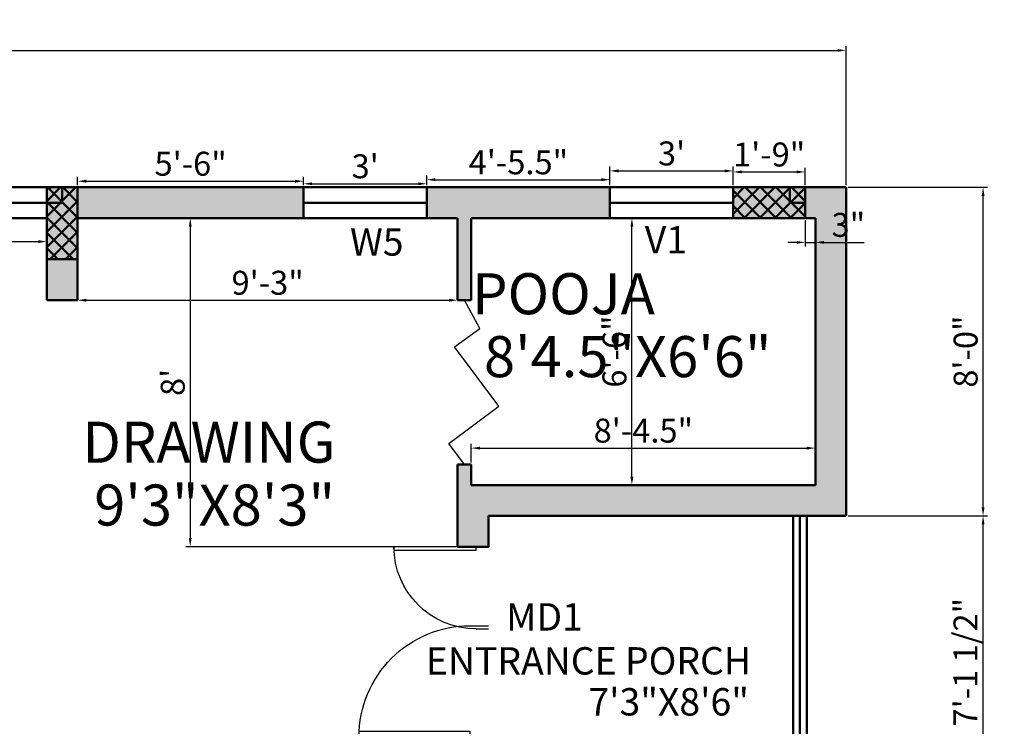
# Model space of a CAD drawing. Units: inches. Extents: x 1749 to 3550, y 1117 to 2383.
# Tile 5 of 15: x 2277 to 2565, y 1481 to 1687. Entities that reach past the tile are written whole.
import ezdxf

# ---------------------------------------------------------------- set-up
doc = ezdxf.new("R2010")
doc.units = ezdxf.units.IN
for name, color, linetype, lineweight in [('A-ANNO-DIMS', 2, 'Continuous', 18), ('A-ANNO-TEXT', 3, 'Continuous', 18), ('A-AREA-IDEN', 7, 'Continuous', 18), ('A-COLS', 10, 'Continuous', 50), ('A-DOOR', 30, 'Continuous', 25), ('A-WALL', 7, 'Continuous', 50), ('A-WALL-PATT', 8, 'Continuous', 13)]:
    doc.layers.add(name, color=color, linetype=linetype, lineweight=lineweight)
doc.styles.get("Standard").update_dxf_attribs({"font": 'arial.ttf'})
doc.dimstyles.new('ISO-25', dxfattribs={"dimtxt": 7, "dimasz": 2.5, "dimexe": 1.25, "dimexo": 0.625, "dimtad": 1, "dimdec": 1, "dimlunit": 3, "dimtxsty": 'Standard', "dimcen": 2.5, "dimadec": 0, "dimazin": 0, "dimtfac": 1, "dimtdec": 1, "dimtmove": 0, "dimatfit": 3, "dimfxl": 1, "dimarcsym": 0})

# ---------------------------------------------------------------- blocks, each defined once
blk = doc.blocks.new('*U14')
for p, q in [((0, 0), (0, 6)), ((36, 0), (36, 6))]:
    blk.add_line(p, q)
blk.add_lwpolyline([(0, 0), (0, -36), (1.75, -36), (1.75, 0)], close=True)
blk.add_arc((0, 0), 36, 270, 0)
blk = doc.blocks.new('*U13')
for p, q in [((0, 0), (0, -6)), ((40, 0), (40, -6))]:
    blk.add_line(p, q)
blk.add_lwpolyline([(0, 0), (0, 40), (1.75, 40), (1.75, 0)], close=True)
blk.add_arc((0, 0), 40, 0, 90)
blk = doc.blocks.new('*D17')
at = {"layer": 'A-ANNO-DIMS', "color": 0, "lineweight": -2, "ltscale": 0.5, "transparency": 16777216}
for p, q in [((2456.64, 1629.24), (2457.26, 1629.24)), ((2456.01, 1553.74), (2456.01, 1626.74)), ((2456.64, 1551.24), (2457.26, 1551.24))]:
    blk.add_line(p, q, dxfattribs=at)
at = {"layer": 'A-ANNO-DIMS', "color": 0, "ltscale": 0.5, "transparency": 16777216}
for points in [[(2455.6, 1626.74), (2456.43, 1626.74), (2456.01, 1629.24)], [(2455.6, 1553.74), (2456.43, 1553.74), (2456.01, 1551.24)]]:
    blk.add_solid(points, dxfattribs=at)
at = {"layer": 'Defpoints', "color": 0, "ltscale": 0.5, "transparency": 16777216}
for p in [(2456.01, 1629.24), (2456.01, 1629.24), (2456.01, 1551.24)]:
    blk.add_point(p, dxfattribs=at)
at = {"layer": 'A-ANNO-DIMS', "color": 0, "ltscale": 0.5, "transparency": 16777216, "insert": (2451.81, 1590.24), "char_height": 7, "attachment_point": 5, "rotation": 90}
blk.add_mtext('6\'-6"', dxfattribs=at)
blk = doc.blocks.new('*D18')
at = {"layer": 'A-ANNO-DIMS', "color": 0, "lineweight": -2, "ltscale": 0.5, "transparency": 16777216}
for p, q in [((2409.1, 1557.87), (2409.1, 1563.29)), ((2411.6, 1562.04), (2507.1, 1562.04)), ((2509.6, 1557.87), (2509.6, 1563.29))]:
    blk.add_line(p, q, dxfattribs=at)
at = {"layer": 'A-ANNO-DIMS', "color": 0, "ltscale": 0.5, "transparency": 16777216}
for points in [[(2411.6, 1562.46), (2411.6, 1561.62), (2409.1, 1562.04)], [(2507.1, 1562.46), (2507.1, 1561.62), (2509.6, 1562.04)]]:
    blk.add_solid(points, dxfattribs=at)
at = {"layer": 'Defpoints', "color": 0, "ltscale": 0.5, "transparency": 16777216}
for p in [(2509.6, 1562.04), (2409.1, 1557.24), (2509.6, 1557.24)]:
    blk.add_point(p, dxfattribs=at)
at = {"layer": 'A-ANNO-DIMS', "color": 0, "ltscale": 0.5, "transparency": 16777216, "insert": (2459.35, 1566.24), "char_height": 7, "attachment_point": 5}
blk.add_mtext('8\'-4.5"', dxfattribs=at)
blk = doc.blocks.new('*D30')
at = {"layer": 'A-ANNO-DIMS', "color": 0, "lineweight": -2, "ltscale": 0.5, "transparency": 16777216}
for p, q in [((2404.48, 1629.24), (2325.74, 1629.24)), ((2326.99, 1626.74), (2326.99, 1535.74)), ((2404.48, 1533.24), (2325.74, 1533.24))]:
    blk.add_line(p, q, dxfattribs=at)
at = {"layer": 'A-ANNO-DIMS', "color": 0, "ltscale": 0.5, "transparency": 16777216}
for points in [[(2326.58, 1626.74), (2327.41, 1626.74), (2326.99, 1629.24)], [(2326.58, 1535.74), (2327.41, 1535.74), (2326.99, 1533.24)]]:
    blk.add_solid(points, dxfattribs=at)
at = {"layer": 'Defpoints', "color": 0, "ltscale": 0.5, "transparency": 16777216}
for p in [(2405.1, 1629.24), (2326.99, 1533.24), (2405.1, 1533.24)]:
    blk.add_point(p, dxfattribs=at)
at = {"layer": 'A-ANNO-DIMS', "color": 0, "ltscale": 0.5, "transparency": 16777216, "insert": (2322.79, 1581.24), "char_height": 7, "attachment_point": 5, "rotation": 90}
blk.add_mtext("8'", dxfattribs=at)
blk = doc.blocks.new('*D31')
at = {"layer": 'A-ANNO-DIMS', "color": 0, "lineweight": -2, "ltscale": 0.5, "transparency": 16777216}
for p, q in [((2294.1, 1605.87), (2294.1, 1606.49)), ((2296.6, 1605.24), (2402.6, 1605.24)), ((2405.1, 1605.87), (2405.1, 1606.49))]:
    blk.add_line(p, q, dxfattribs=at)
at = {"layer": 'A-ANNO-DIMS', "color": 0, "ltscale": 0.5, "transparency": 16777216}
for points in [[(2296.6, 1605.66), (2296.6, 1604.83), (2294.1, 1605.24)], [(2402.6, 1605.66), (2402.6, 1604.83), (2405.1, 1605.24)]]:
    blk.add_solid(points, dxfattribs=at)
at = {"layer": 'Defpoints', "color": 0, "ltscale": 0.5, "transparency": 16777216}
for p in [(2294.1, 1605.24), (2405.1, 1605.24), (2405.1, 1605.24)]:
    blk.add_point(p, dxfattribs=at)
at = {"layer": 'A-ANNO-DIMS', "color": 0, "ltscale": 0.5, "transparency": 16777216, "insert": (2349.6, 1609.44), "char_height": 7, "attachment_point": 5}
blk.add_mtext('9\'-3"', dxfattribs=at)
blk = doc.blocks.new('*D36')
at = {"layer": 'A-ANNO-DIMS', "color": 0, "lineweight": -2, "ltscale": 0.5, "transparency": 16777216}
for p, q in [((2113.1, 1628.62), (2113.1, 1621.13)), ((2285.1, 1628.62), (2285.1, 1621.13)), ((2115.6, 1622.38), (2282.6, 1622.38))]:
    blk.add_line(p, q, dxfattribs=at)
at = {"layer": 'A-ANNO-DIMS', "color": 0, "ltscale": 0.5, "transparency": 16777216}
for points in [[(2115.6, 1622.8), (2115.6, 1621.97), (2113.1, 1622.38)], [(2282.6, 1622.8), (2282.6, 1621.97), (2285.1, 1622.38)]]:
    blk.add_solid(points, dxfattribs=at)
at = {"layer": 'Defpoints', "color": 0, "ltscale": 0.5, "transparency": 16777216}
for p in [(2113.1, 1629.24), (2285.1, 1629.24), (2285.1, 1622.38)]:
    blk.add_point(p, dxfattribs=at)
at = {"layer": 'A-ANNO-DIMS', "color": 0, "ltscale": 0.5, "transparency": 16777216, "insert": (2199.1, 1626.52), "char_height": 7, "attachment_point": 5}
blk.add_mtext('14\'-4"', dxfattribs=at)
blk = doc.blocks.new('*D37')
at = {"layer": 'A-ANNO-DIMS', "color": 0, "lineweight": -2, "ltscale": 0.5, "transparency": 16777216}
for p, q in [((2294.1, 1638.87), (2294.1, 1641.27)), ((2296.6, 1640.02), (2357.6, 1640.02)), ((2360.1, 1638.87), (2360.1, 1641.27))]:
    blk.add_line(p, q, dxfattribs=at)
at = {"layer": 'A-ANNO-DIMS', "color": 0, "ltscale": 0.5, "transparency": 16777216}
for points in [[(2296.6, 1640.44), (2296.6, 1639.6), (2294.1, 1640.02)], [(2357.6, 1640.44), (2357.6, 1639.6), (2360.1, 1640.02)]]:
    blk.add_solid(points, dxfattribs=at)
at = {"layer": 'Defpoints', "color": 0, "ltscale": 0.5, "transparency": 16777216}
for p in [(2360.1, 1640.02), (2294.1, 1638.24), (2360.1, 1638.24)]:
    blk.add_point(p, dxfattribs=at)
at = {"layer": 'A-ANNO-DIMS', "color": 0, "ltscale": 0.5, "transparency": 16777216, "insert": (2327.1, 1644.22), "char_height": 7, "attachment_point": 5}
blk.add_mtext('5\'-6"', dxfattribs=at)
blk = doc.blocks.new('*D38')
at = {"layer": 'A-ANNO-DIMS', "color": 0, "lineweight": -2, "ltscale": 0.5, "transparency": 16777216}
for p, q in [((2360.1, 1638.87), (2360.1, 1640.52)), ((2396.1, 1638.87), (2396.1, 1640.52)), ((2362.6, 1639.27), (2393.6, 1639.27))]:
    blk.add_line(p, q, dxfattribs=at)
at = {"layer": 'A-ANNO-DIMS', "color": 0, "ltscale": 0.5, "transparency": 16777216}
for points in [[(2362.6, 1639.68), (2362.6, 1638.85), (2360.1, 1639.27)], [(2393.6, 1639.68), (2393.6, 1638.85), (2396.1, 1639.27)]]:
    blk.add_solid(points, dxfattribs=at)
at = {"layer": 'Defpoints', "color": 0, "ltscale": 0.5, "transparency": 16777216}
for p in [(2360.1, 1638.24), (2396.1, 1639.27), (2396.1, 1638.24)]:
    blk.add_point(p, dxfattribs=at)
at = {"layer": 'A-ANNO-DIMS', "color": 0, "ltscale": 0.5, "transparency": 16777216, "insert": (2378.1, 1643.47), "char_height": 7, "attachment_point": 5}
blk.add_mtext("3'", dxfattribs=at)
blk = doc.blocks.new('*D39')
at = {"layer": 'A-ANNO-DIMS', "color": 0, "lineweight": -2, "ltscale": 0.5, "transparency": 16777216}
for p, q in [((2396.1, 1638.87), (2396.1, 1641.71)), ((2398.6, 1640.46), (2447.1, 1640.46)), ((2449.6, 1638.87), (2449.6, 1641.71))]:
    blk.add_line(p, q, dxfattribs=at)
at = {"layer": 'A-ANNO-DIMS', "color": 0, "ltscale": 0.5, "transparency": 16777216}
for points in [[(2398.6, 1640.87), (2398.6, 1640.04), (2396.1, 1640.46)], [(2447.1, 1640.87), (2447.1, 1640.04), (2449.6, 1640.46)]]:
    blk.add_solid(points, dxfattribs=at)
at = {"layer": 'Defpoints', "color": 0, "ltscale": 0.5, "transparency": 16777216}
for p in [(2449.6, 1640.46), (2396.1, 1638.24), (2449.6, 1638.24)]:
    blk.add_point(p, dxfattribs=at)
at = {"layer": 'A-ANNO-DIMS', "color": 0, "ltscale": 0.5, "transparency": 16777216, "insert": (2422.85, 1644.64), "char_height": 7, "attachment_point": 5}
blk.add_mtext('4\'-5.5"', dxfattribs=at)
blk = doc.blocks.new('*D40')
at = {"layer": 'A-ANNO-DIMS', "color": 0, "lineweight": -2, "ltscale": 0.5, "transparency": 16777216}
for p, q in [((2449.6, 1638.87), (2449.6, 1644.28)), ((2452.1, 1643.03), (2483.1, 1643.03)), ((2485.6, 1638.87), (2485.6, 1644.28))]:
    blk.add_line(p, q, dxfattribs=at)
at = {"layer": 'A-ANNO-DIMS', "color": 0, "ltscale": 0.5, "transparency": 16777216}
for points in [[(2452.1, 1643.45), (2452.1, 1642.61), (2449.6, 1643.03)], [(2483.1, 1643.45), (2483.1, 1642.61), (2485.6, 1643.03)]]:
    blk.add_solid(points, dxfattribs=at)
at = {"layer": 'Defpoints', "color": 0, "ltscale": 0.5, "transparency": 16777216}
for p in [(2485.6, 1643.03), (2449.6, 1638.24), (2485.6, 1638.24)]:
    blk.add_point(p, dxfattribs=at)
at = {"layer": 'A-ANNO-DIMS', "color": 0, "ltscale": 0.5, "transparency": 16777216, "insert": (2467.6, 1647.23), "char_height": 7, "attachment_point": 5}
blk.add_mtext("3'", dxfattribs=at)
blk = doc.blocks.new('*D41')
at = {"layer": 'A-ANNO-DIMS', "color": 0, "lineweight": -2, "ltscale": 0.5, "transparency": 16777216}
for p, q in [((2485.6, 1638.87), (2485.6, 1643.97)), ((2488.1, 1642.72), (2504.1, 1642.72)), ((2506.6, 1638.87), (2506.6, 1643.97))]:
    blk.add_line(p, q, dxfattribs=at)
at = {"layer": 'A-ANNO-DIMS', "color": 0, "ltscale": 0.5, "transparency": 16777216}
for points in [[(2488.1, 1643.14), (2488.1, 1642.31), (2485.6, 1642.72)], [(2504.1, 1643.14), (2504.1, 1642.31), (2506.6, 1642.72)]]:
    blk.add_solid(points, dxfattribs=at)
at = {"layer": 'Defpoints', "color": 0, "ltscale": 0.5, "transparency": 16777216}
for p in [(2506.6, 1642.72), (2485.6, 1638.24), (2506.6, 1638.24)]:
    blk.add_point(p, dxfattribs=at)
at = {"layer": 'A-ANNO-DIMS', "color": 0, "ltscale": 0.5, "transparency": 16777216, "insert": (2496.1, 1646.92), "char_height": 7, "attachment_point": 5}
blk.add_mtext('1\'-9"', dxfattribs=at)
blk = doc.blocks.new('*D42')
at = {"layer": 'A-ANNO-DIMS', "color": 0, "lineweight": -2, "ltscale": 0.5, "transparency": 16777216}
for p, q in [((2506.6, 1628.62), (2506.6, 1620.9)), ((2509.6, 1628.62), (2509.6, 1620.9)), ((2504.1, 1622.15), (2501.6, 1622.15)), ((2506.6, 1622.15), (2509.6, 1622.15)), ((2512.1, 1622.15), (2523.9, 1622.15))]:
    blk.add_line(p, q, dxfattribs=at)
at = {"layer": 'A-ANNO-DIMS', "color": 0, "ltscale": 0.5, "transparency": 16777216}
for points in [[(2504.1, 1622.57), (2504.1, 1621.73), (2506.6, 1622.15)], [(2512.1, 1622.57), (2512.1, 1621.73), (2509.6, 1622.15)]]:
    blk.add_solid(points, dxfattribs=at)
at = {"layer": 'Defpoints', "color": 0, "ltscale": 0.5, "transparency": 16777216}
for p in [(2506.6, 1629.24), (2509.6, 1629.24), (2509.6, 1622.15)]:
    blk.add_point(p, dxfattribs=at)
at = {"layer": 'A-ANNO-DIMS', "color": 0, "ltscale": 0.5, "transparency": 16777216, "insert": (2519.25, 1626.35), "char_height": 7, "attachment_point": 5}
blk.add_mtext('3"', dxfattribs=at)
blk = doc.blocks.new('*D172')
at = {"layer": 'A-ANNO-DIMS', "color": 0, "lineweight": -2, "ltscale": 0.5, "transparency": 16777216}
for p, q in [((1859.6, 1638.87), (1859.6, 1679.49)), ((1862.1, 1678.24), (2516.1, 1678.24)), ((2518.6, 1638.87), (2518.6, 1679.49))]:
    blk.add_line(p, q, dxfattribs=at)
at = {"layer": 'A-ANNO-DIMS', "color": 0, "ltscale": 0.5, "transparency": 16777216}
for points in [[(1862.1, 1678.66), (1862.1, 1677.83), (1859.6, 1678.24)], [(2516.1, 1678.66), (2516.1, 1677.83), (2518.6, 1678.24)]]:
    blk.add_solid(points, dxfattribs=at)
at = {"layer": 'Defpoints', "color": 0, "ltscale": 0.5, "transparency": 16777216}
for p in [(2518.6, 1678.24), (1859.6, 1638.24), (2518.6, 1638.24)]:
    blk.add_point(p, dxfattribs=at)
at = {"layer": 'A-ANNO-DIMS', "color": 0, "ltscale": 0.5, "transparency": 16777216, "insert": (2189.1, 1682.44), "char_height": 7, "attachment_point": 5}
blk.add_mtext('54\'-11"', dxfattribs=at)
blk = doc.blocks.new('*D174')
at = {"layer": 'A-ANNO-DIMS', "color": 0, "lineweight": -2, "ltscale": 0.5, "transparency": 16777216}
for p, q in [((2519.23, 1542.24), (2559.85, 1542.24)), ((2558.6, 1459.24), (2558.6, 1539.74)), ((2414.73, 1456.74), (2559.85, 1456.74))]:
    blk.add_line(p, q, dxfattribs=at)
at = {"layer": 'A-ANNO-DIMS', "color": 0, "ltscale": 0.5, "transparency": 16777216}
for points in [[(2558.19, 1539.74), (2559.02, 1539.74), (2558.6, 1542.24)], [(2558.19, 1459.24), (2559.02, 1459.24), (2558.6, 1456.74)]]:
    blk.add_solid(points, dxfattribs=at)
at = {"layer": 'Defpoints', "color": 0, "ltscale": 0.5, "transparency": 16777216}
for p in [(2518.6, 1542.24), (2558.6, 1542.24), (2414.1, 1456.74)]:
    blk.add_point(p, dxfattribs=at)
at = {"layer": 'A-ANNO-DIMS', "color": 0, "ltscale": 0.5, "transparency": 16777216, "insert": (2554.36, 1499.49), "char_height": 7, "attachment_point": 5, "rotation": 90}
blk.add_mtext('7\'-1 1/2"', dxfattribs=at)
blk = doc.blocks.new('*D175')
at = {"layer": 'A-ANNO-DIMS', "color": 0, "lineweight": -2, "ltscale": 0.5, "transparency": 16777216}
for p, q in [((2519.23, 1638.24), (2559.85, 1638.24)), ((2558.6, 1544.74), (2558.6, 1635.74)), ((2519.23, 1542.24), (2559.85, 1542.24))]:
    blk.add_line(p, q, dxfattribs=at)
at = {"layer": 'A-ANNO-DIMS', "color": 0, "ltscale": 0.5, "transparency": 16777216}
for points in [[(2558.19, 1635.74), (2559.02, 1635.74), (2558.6, 1638.24)], [(2558.19, 1544.74), (2559.02, 1544.74), (2558.6, 1542.24)]]:
    blk.add_solid(points, dxfattribs=at)
at = {"layer": 'Defpoints', "color": 0, "ltscale": 0.5, "transparency": 16777216}
for p in [(2518.6, 1638.24), (2558.6, 1638.24), (2518.6, 1542.24)]:
    blk.add_point(p, dxfattribs=at)
at = {"layer": 'A-ANNO-DIMS', "color": 0, "ltscale": 0.5, "transparency": 16777216, "insert": (2554.41, 1590.24), "char_height": 7, "attachment_point": 5, "rotation": 90}
blk.add_mtext('8\'-0"', dxfattribs=at)

msp = doc.modelspace()

# ---------------------------------------------------------------- hatches: boundary and pattern name
at = {"layer": 'A-COLS', "ltscale": 10}
h = msp.add_hatch(color=256, dxfattribs=at)
h.dxf.hatch_style = 1
h.paths.add_polyline_path([(2285.1, 1638.24), (2285.1, 1633.74), (2289.6, 1633.74), (2289.6, 1638.24)])
h = msp.add_hatch(dxfattribs=at)
h.set_pattern_fill('ANSI37', color=256, angle=90)
h.set_pattern_definition([(135, (3652.2103, -34.0015), (-2.245064, -2.245064), []), (225, (3652.2103, -34.0015), (2.245064, -2.245064), [])])
h.paths.add_polyline_path([(2294.1, 1638.24), (2285.1, 1638.24), (2285.1, 1617.24), (2294.1, 1617.24)])
h = msp.add_hatch(dxfattribs=at)
h.set_pattern_fill('ANSI37', color=256)
h.set_pattern_definition([(45, (834.36, 271.1368), (-2.245064, 2.245064), []), (135, (834.36, 271.1368), (-2.245064, -2.245064), [])])
h.paths.add_polyline_path([(2506.6, 1629.24), (2506.6, 1638.24), (2485.6, 1638.24), (2485.6, 1629.24)])
h = msp.add_hatch(color=256, dxfattribs=at)
h.dxf.hatch_style = 1
h.paths.add_polyline_path([(2502.1, 1638.24), (2502.1, 1633.74), (2506.6, 1633.74), (2506.6, 1638.24)])
at = {"layer": 'A-WALL-PATT', "ltscale": 10}
h = msp.add_hatch(color=256, dxfattribs=at)
h.dxf.hatch_style = 1
h.paths.add_polyline_path([(2285.1, 1638.24), (2285.1, 1629.24), (2285.1, 1605.24), (2294.1, 1605.24), (2294.1, 1629.24), (2360.1, 1629.24), (2360.1, 1638.24)])
h = msp.add_hatch(color=256, dxfattribs=at)
h.dxf.hatch_style = 1
h.paths.add_polyline_path([(2449.6, 1629.24), (2449.6, 1638.24), (2396.1, 1638.24), (2396.1, 1629.24), (2405.1, 1629.24), (2405.1, 1605.24), (2409.1, 1605.24), (2409.1, 1629.24)])
h = msp.add_hatch(color=256, dxfattribs=at)
h.dxf.hatch_style = 1
h.paths.add_polyline_path([(2509.6, 1629.24), (2509.6, 1551.24), (2409.1, 1551.24), (2409.1, 1557.24), (2405.1, 1557.24), (2405.1, 1533.24), (2414.1, 1533.24), (2414.1, 1542.24), (2498.1, 1542.24), (2503.1, 1542.24), (2507.1, 1542.24), (2518.6, 1542.24), (2518.6, 1638.24), (2485.6, 1638.24), (2485.6, 1629.24)])

# ---------------------------------------------------------------- linework, layer by layer
at = {"layer": 'A-COLS', "ltscale": 10}
for points in [[(2285.1, 1638.24), (2289.6, 1638.24), (2289.6, 1633.74), (2285.1, 1633.74)], [(2285.1, 1617.24), (2285.1, 1638.24), (2294.1, 1638.24), (2294.1, 1617.24)], [(2485.6, 1638.24), (2506.6, 1638.24), (2506.6, 1629.24), (2485.6, 1629.24)], [(2502.1, 1638.24), (2506.6, 1638.24), (2506.6, 1633.74), (2502.1, 1633.74)]]:
    msp.add_lwpolyline(points, close=True, dxfattribs=at)
at = {"layer": 'A-DOOR', "ltscale": 0.5}
for p, q in [((2411.58, 1596.99), (2407.1, 1605.24)), ((2404.17, 1591.65), (2411.58, 1596.99)), ((2417.1, 1574.29), (2404.17, 1591.65)), ((2402.5, 1563.42), (2417.1, 1574.29)), ((2407.1, 1557.24), (2402.5, 1563.42))]:
    msp.add_line(p, q, dxfattribs=at)
at = {"layer": 'A-WALL', "ltscale": 0.2}
for p, q in [((1859.6, 1638.24), (2518.6, 1638.24)), ((2285.1, 1629.24), (2285.1, 1638.24)), ((2360.1, 1629.24), (2360.1, 1638.24)), ((2396.1, 1629.24), (2396.1, 1638.24)), ((2449.6, 1629.24), (2449.6, 1638.24)), ((2485.6, 1629.24), (2485.6, 1638.24)), ((2518.6, 1638.24), (2518.6, 1542.24)), ((2360.1, 1633.74), (2396.1, 1633.74)), ((2449.6, 1633.74), (2485.6, 1633.74)), ((2113.1, 1629.24), (2285.1, 1629.24)), ((2285.1, 1605.24), (2285.1, 1629.24)), ((2294.1, 1629.24), (2294.1, 1605.24)), ((2294.1, 1629.24), (2405.1, 1629.24)), ((2405.1, 1629.24), (2405.1, 1605.24)), ((2409.1, 1629.24), (2409.1, 1605.24)), ((2409.1, 1629.24), (2509.6, 1629.24)), ((2509.6, 1629.24), (2509.6, 1551.24)), ((2285.1, 1605.24), (2294.1, 1605.24)), ((2409.1, 1605.24), (2405.1, 1605.24)), ((2409.1, 1557.24), (2405.1, 1557.24)), ((2405.1, 1557.24), (2405.1, 1533.24)), ((2409.1, 1557.24), (2409.1, 1551.24)), ((2409.1, 1551.24), (2509.6, 1551.24)), ((2414.1, 1542.24), (2498.1, 1542.24)), ((2414.1, 1542.24), (2414.1, 1533.24)), ((2498.1, 1542.24), (2503.1, 1542.24)), ((2503.1, 1403.24), (2503.1, 1542.24)), ((2503.1, 1542.24), (2507.1, 1542.24)), ((2505.1, 1454.24), (2505.1, 1542.24)), ((2507.1, 1542.24), (2507.1, 1367.24)), ((2507.1, 1542.24), (2518.6, 1542.24)), ((2414.1, 1533.24), (2405.1, 1533.24))]:
    msp.add_line(p, q, dxfattribs=at)
at = {"layer": 'A-WALL', "ltscale": 0.5}
msp.add_line((2285.1, 1633.74), (2113.1, 1633.74), dxfattribs=at)

# ---------------------------------------------------------------- block references
at = {"layer": 'A-DOOR'}
for name, p, xscale, yscale, zscale, rotation in [('*U13', (2410.5, 1533.24), -0.6, 0.6, 0.6, 90), ('*U14', (2408.7, 1477.74), -0.9, 0.9, 0.9, 270)]:
    msp.add_blockref(name, p, dxfattribs=dict(at, xscale=xscale, yscale=yscale, zscale=zscale, rotation=rotation))

# ---------------------------------------------------------------- texts
at = {"layer": 'A-ANNO-TEXT', "ltscale": 0.5}
for s, p in [('W5', (2373.67, 1618.27)), ('V1', (2459.76, 1618.92)), ('MD1', (2419.26, 1508.72))]:
    msp.add_text(s, height=8, dxfattribs=at).set_placement(p)
at = {"layer": 'A-AREA-IDEN', "ltscale": 0.5}
for s, height, p in [('POOJA', 12, (2409.34, 1601.12)), ('DRAWING', 12, (2295.48, 1557.75)), ('ENTRANCE PORCH', 8, (2395.85, 1495.85))]:
    msp.add_text(s, height=height, rotation=0.0333, dxfattribs=at).set_placement(p)
for s, height, p in [('8\'4.5"X6\'6"', 12, (2412.8, 1582.77)), ('9\'3"X8\'3"', 12, (2298.95, 1539.4)), ('7\'3"X8\'6"', 8, (2443.31, 1483.91))]:
    msp.add_text(s, height=height, dxfattribs=at).set_placement(p)

# ---------------------------------------------------------------- dimensions: what is measured, and where the dimension line sits
at = {"layer": 'A-ANNO-DIMS', "ltscale": 0.5}
for base, p1, p2, override, picture, middle in [((2518.6, 1678.24), (1859.6, 1638.24), (2518.6, 1638.24), {"dimdec": 1, "dimlfac": 1, "dimrnd": 0, "dimzin": 1, "dimdsep": 46, "dimlunit": 4, "dimfrac": 2}, '*D172', (2189.1, 1682.44)), ((2485.6, 1643.03), (2449.6, 1638.24), (2485.6, 1638.24), {"dimclrd": 0, "dimclre": 0, "dimclrt": 0}, '*D40', (2467.6, 1647.23)), ((2506.6, 1642.72), (2485.6, 1638.24), (2506.6, 1638.24), {"dimclrd": 0, "dimclre": 0, "dimclrt": 0}, '*D41', (2496.1, 1646.92)), ((2360.1, 1640.02), (2294.1, 1638.24), (2360.1, 1638.24), {"dimclrd": 0, "dimclre": 0, "dimclrt": 0}, '*D37', (2327.1, 1644.22)), ((2396.1, 1639.27), (2360.1, 1638.24), (2396.1, 1638.24), {"dimclrd": 0, "dimclre": 0, "dimclrt": 0}, '*D38', (2378.1, 1643.47)), ((2449.6, 1640.46), (2396.1, 1638.24), (2449.6, 1638.24), {"dimclrd": 0, "dimclre": 0, "dimclrt": 0}, '*D39', (2422.85, 1644.64)), ((2285.1, 1622.38), (2113.1, 1629.24), (2285.1, 1629.24), {"dimclrd": 0, "dimclre": 0, "dimclrt": 0}, '*D36', (2199.1, 1626.52)), ((2509.6, 1622.15), (2506.6, 1629.24), (2509.6, 1629.24), {"dimclrd": 0, "dimclre": 0, "dimclrt": 0}, '*D42', (2519.25, 1626.35)), ((2405.1, 1605.24), (2294.1, 1605.24), (2405.1, 1605.24), {"dimclrd": 0, "dimclre": 0, "dimclrt": 0}, '*D31', (2349.6, 1609.44)), ((2509.6, 1562.04), (2409.1, 1557.24), (2509.6, 1557.24), {"dimclrd": 0, "dimclre": 0, "dimclrt": 0}, '*D18', (2459.35, 1566.24))]:
    dim = msp.add_linear_dim(base=base, p1=p1, p2=p2, dimstyle='ISO-25', override=override, dxfattribs=at)
    dim.commit()
    dim.dimension.update_dxf_attribs({"geometry": picture, "text_midpoint": middle})
for base, p1, p2, override, picture, middle in [((2558.6, 1638.24), (2518.6, 1542.24), (2518.6, 1638.24), {"dimdec": 1, "dimlfac": 1, "dimrnd": 0, "dimzin": 1, "dimdsep": 46, "dimlunit": 4, "dimfrac": 2}, '*D175', (2554.41, 1590.24)), ((2326.99, 1533.24), (2405.1, 1629.24), (2405.1, 1533.24), {"dimclrd": 0, "dimclre": 0, "dimclrt": 0}, '*D30', (2322.79, 1581.24)), ((2456.01, 1629.24), (2456.01, 1551.24), (2456.01, 1629.24), {"dimclrd": 0, "dimclre": 0, "dimclrt": 0}, '*D17', (2451.81, 1590.24)), ((2558.6, 1542.24), (2414.1, 1456.74), (2518.6, 1542.24), {"dimdec": 1, "dimlfac": 1, "dimrnd": 0, "dimzin": 1, "dimdsep": 46, "dimlunit": 4, "dimfrac": 2}, '*D174', (2554.36, 1499.49))]:
    dim = msp.add_linear_dim(base=base, p1=p1, p2=p2, angle=90, dimstyle='ISO-25', override=override, dxfattribs=at)
    dim.commit()
    dim.dimension.update_dxf_attribs({"geometry": picture, "text_midpoint": middle})

doc.saveas('drawing.dxf')
